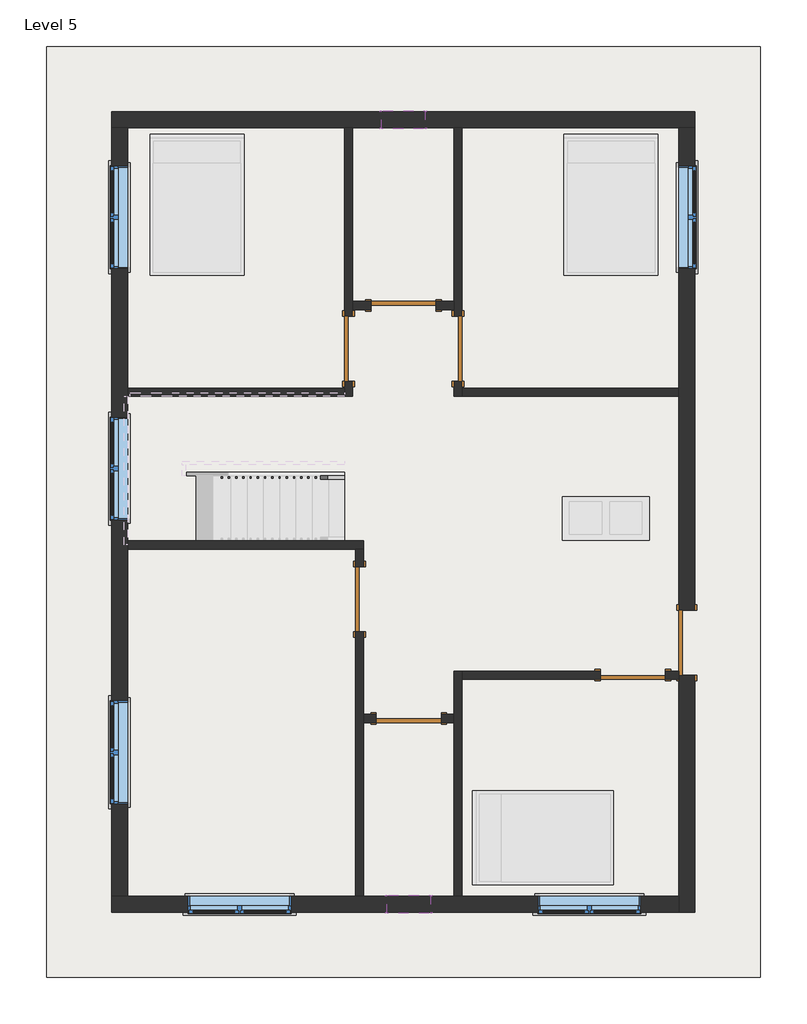
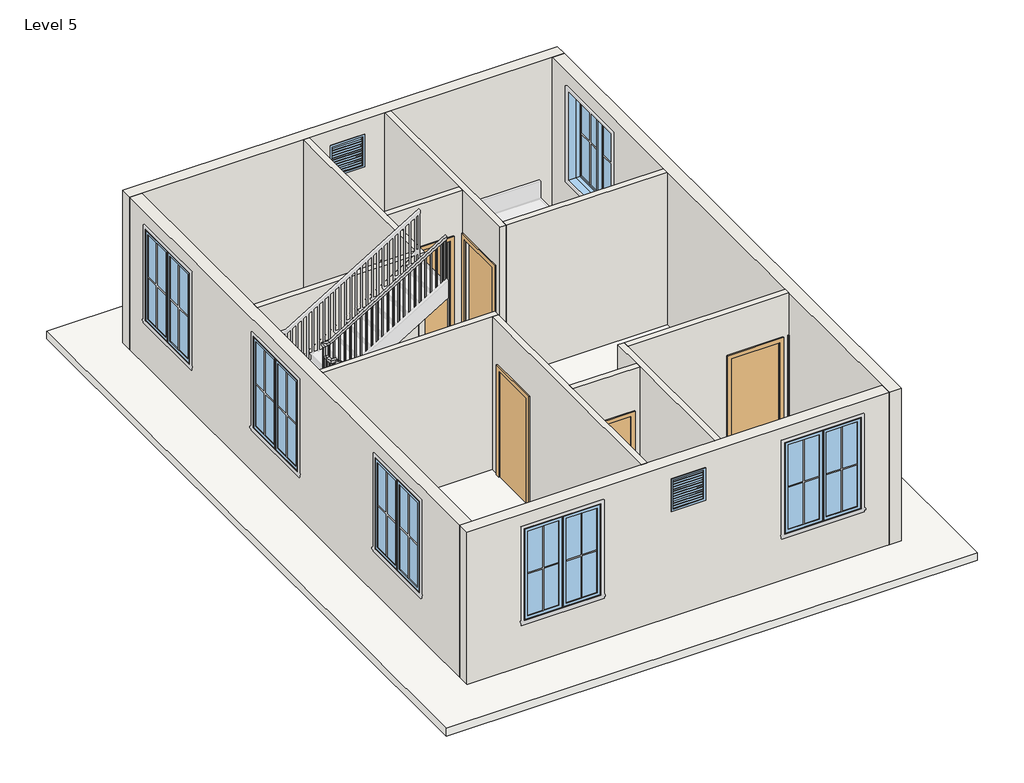
# One storey, part 1 of 2: 14 walls, 8 windows, 7 doors, 1 railing, 1 roof, 1 slab.
"""IFC4 building model written with IfcOpenShell, lengths in millimetres."""

from ifc_helpers import new_model, si_unit, frame, origin, place, context, project, spatial, polyline, outline, extrude, faceted_brep, transform, mapped, element, save
from components import door_305aa2a5, door_e5f9f3c4, door_0ca8825f, window_9ac97e1a, window_f2d8fef0

model = new_model("IFC4")

# Units and contexts
model_context = context("Model", 3, world=origin())
ifc_project = project(units=[si_unit("LENGTHUNIT", "METRE", prefix="MILLI")], contexts=[model_context])

# Site, building, storey
site = spatial("IfcSite", under=ifc_project)
building = spatial("IfcBuilding", under=site)
storey = spatial("IfcBuildingStorey", under=building, Name="Level 5", Elevation=9601.2)

# Doors
placement = place(None, origin())
door_shape = door_305aa2a5(model_context)
element("IfcDoor", 1, ObjectType="Single-Flush : 36\" x 84\"", at=placement, inside=storey, context=model_context, shape_type="MappedRepresentation", body=[
    mapped(door_shape, transform((-2023.6910855, 2116.5303617, 9601.2), x_axis=(0.0, -1.0, 0.0), y_axis=(1.0, 0.0, 0.0), z_axis=(0.0, 0.0, 1.0))),
])
element("IfcDoor", 2, ObjectType="Single-Flush : 36\" x 84\"", at=placement, inside=storey, context=model_context, shape_type="MappedRepresentation", body=[
    mapped(door_shape, transform((-1179.1410855, -3078.1725945, 9601.2), x_axis=(1.0, 0.0, 0.0), y_axis=(0.0, 1.0, 0.0), z_axis=(0.0, 0.0, 1.0))),
])
element("IfcDoor", 3, ObjectType="Single-Flush : 36\" x 84\"", at=placement, inside=storey, context=model_context, shape_type="MappedRepresentation", body=[
    mapped(door_shape, transform((1970.4589145, -2468.1696383, 9601.2), x_axis=(1.0, 0.0, 0.0), y_axis=(0.0, 1.0, 0.0), z_axis=(0.0, 0.0, 1.0))),
])
door_2_shape = door_e5f9f3c4(model_context)
element("IfcDoor", 4, ObjectType="Single-Flush : 36\" x 84\"", at=placement, inside=storey, context=model_context, shape_type="MappedRepresentation", body=[
    mapped(door_2_shape, transform((-486.9910855, 2116.5303617, 9601.2), x_axis=(0.0, -1.0, 0.0), y_axis=(1.0, 0.0, 0.0), z_axis=(0.0, 0.0, 1.0))),
])
element("IfcDoor", 5, ObjectType="Single-Flush : 36\" x 84\"", at=placement, inside=storey, context=model_context, shape_type="MappedRepresentation", body=[
    mapped(door_2_shape, transform((-1871.2910855, -1401.3696383, 9601.2), x_axis=(0.0, 1.0, 0.0), y_axis=(-1.0, 0.0, 0.0), z_axis=(0.0, 0.0, 1.0))),
])
element("IfcDoor", 6, ObjectType="Single-Flush : 36\" x 84\"", at=placement, inside=storey, context=model_context, shape_type="MappedRepresentation", body=[
    mapped(door_2_shape, transform((-1255.3410855, 2726.1303617, 9601.2), x_axis=(1.0, 0.0, 0.0), y_axis=(0.0, 1.0, 0.0), z_axis=(0.0, 0.0, 1.0))),
])
door_3_shape = door_0ca8825f(model_context)
element("IfcDoor", 7, ObjectType="Single-Flush : 36\" x 84\"", at=placement, inside=storey, context=model_context, shape_type="MappedRepresentation", body=[
    mapped(door_3_shape, transform((2732.4589145, -2010.9696383, 9601.2), x_axis=(0.0, 1.0, 0.0), y_axis=(-1.0, 0.0, 0.0), z_axis=(0.0, 0.0, 1.0))),
])

# Railing
element("IfcRailing", 8, ObjectType="Handrail - Rectangular", at=placement, inside=storey, context=model_context, shape_type="SolidModel", body=[
    faceted_brep([(-2080.8410855, 281.3803617, 10654.1454545), (-2080.8410855, 281.3803617, 10594.7439943), (-2080.8410855, 332.1803617, 10594.7439943), (-2080.8410855, 332.1803617, 10654.1454545), (-4290.6410855, 281.3803617, 11993.4181818), (-4341.4410855, 281.3803617, 11964.8046004), (-4341.4410855, 332.1803617, 11964.8046004), (-4290.6410855, 332.1803617, 11993.4181818), (-4290.6410855, 281.3803617, 12039.6), (-4341.4410855, 281.3803617, 11988.8), (-4341.4410855, 332.1803617, 11988.8), (-4290.6410855, 332.1803617, 12039.6), (-4417.6410855, 281.3803617, 12039.6), (-4417.6410855, 281.3803617, 11988.8), (-4366.8410855, 332.1803617, 11988.8), (-4366.8410855, 332.1803617, 12039.6), (-4417.6410855, 408.3803617, 12039.6), (-4417.6410855, 408.3803617, 11988.8), (-4366.8410855, 408.3803617, 11988.8), (-4366.8410855, 408.3803617, 12039.6), (-4417.6410855, 459.1803617, 12039.6), (-4417.6410855, 509.9803617, 11988.8), (-4366.8410855, 509.9803617, 11988.8), (-4366.8410855, 459.1803617, 12039.6), (-4417.6410855, 459.1803617, 12224.3272727), (-4417.6410855, 509.9803617, 12173.5272727), (-4366.8410855, 509.9803617, 12173.5272727), (-4366.8410855, 459.1803617, 12224.3272727), (-4417.6410855, 586.1803617, 12224.3272727), (-4417.6410855, 586.1803617, 12173.5272727), (-4366.8410855, 535.3803617, 12173.5272727), (-4366.8410855, 535.3803617, 12224.3272727), (-4290.6410855, 586.1803617, 12224.3272727), (-4276.4486761, 586.1803617, 12173.5272727), (-4276.4486761, 535.3803617, 12173.5272727), (-4290.6410855, 535.3803617, 12224.3272727), (-2080.8410855, 586.1803617, 13563.6), (-2080.8410855, 535.3803617, 13563.6), (-2080.8410855, 535.3803617, 13504.1985397), (-2080.8410855, 586.1803617, 13504.1985397)], [[[0, 1, 2, 3]], [[1, 0, 4, 5]], [[2, 1, 5, 6]], [[3, 2, 6, 7]], [[0, 3, 7, 4]], [[5, 4, 8, 9]], [[6, 5, 9, 10]], [[7, 6, 10, 11]], [[4, 7, 11, 8]], [[9, 8, 12, 13]], [[10, 9, 13, 14]], [[11, 10, 14, 15]], [[8, 11, 15, 12]], [[13, 12, 16, 17]], [[14, 13, 17, 18]], [[15, 14, 18, 19]], [[12, 15, 19, 16]], [[17, 16, 20, 21]], [[18, 17, 21, 22]], [[19, 18, 22, 23]], [[16, 19, 23, 20]], [[21, 20, 24, 25]], [[22, 21, 25, 26]], [[23, 22, 26, 27]], [[20, 23, 27, 24]], [[25, 24, 28, 29]], [[26, 25, 29, 30]], [[27, 26, 30, 31]], [[24, 27, 31, 28]], [[29, 28, 32, 33]], [[30, 29, 33, 34]], [[31, 30, 34, 35]], [[28, 31, 35, 32]], [[36, 37, 38, 39]], [[33, 32, 36, 39]], [[34, 33, 39, 38]], [[35, 34, 38, 37]], [[32, 35, 37, 36]]]),
    extrude(outline(polyline([(13463.7894488, -2147.5160855), (13452.2439943, -2166.5660855), (12510.6545455, -2166.5660855), (12510.6545455, -2147.5160855), (13463.7894488, -2147.5160855)])), frame((0.0, 551.2553617, 0.0), z_axis=(0.0, 1.0, 0.0), x_axis=(0.0, 0.0, 1.0)), (0.0, 0.0, 1.0), 19.05),
    extrude(outline(polyline([(13402.2136913, -2249.1160855), (13390.6682367, -2268.1660855), (12510.6545455, -2268.1660855), (12510.6545455, -2249.1160855), (13402.2136913, -2249.1160855)])), frame((0.0, 551.2553617, 0.0), z_axis=(0.0, 1.0, 0.0), x_axis=(0.0, 0.0, 1.0)), (0.0, 0.0, 1.0), 19.05),
    extrude(outline(polyline([(13340.6379337, -2350.7160855), (13329.0924791, -2369.7660855), (12372.1090909, -2369.7660855), (12372.1090909, -2350.7160855), (13340.6379337, -2350.7160855)])), frame((0.0, 551.2553617, 0.0), z_axis=(0.0, 1.0, 0.0), x_axis=(0.0, 0.0, 1.0)), (0.0, 0.0, 1.0), 19.05),
    extrude(outline(polyline([(13279.0621761, -2452.3160855), (13267.5167216, -2471.3660855), (12372.1090909, -2471.3660855), (12372.1090909, -2452.3160855), (13279.0621761, -2452.3160855)])), frame((0.0, 551.2553617, 0.0), z_axis=(0.0, 1.0, 0.0), x_axis=(0.0, 0.0, 1.0)), (0.0, 0.0, 1.0), 19.05),
    extrude(outline(polyline([(13217.4864185, -2553.9160855), (13205.940964, -2572.9660855), (12233.5636364, -2572.9660855), (12233.5636364, -2553.9160855), (13217.4864185, -2553.9160855)])), frame((0.0, 551.2553617, 0.0), z_axis=(0.0, 1.0, 0.0), x_axis=(0.0, 0.0, 1.0)), (0.0, 0.0, 1.0), 19.05),
    extrude(outline(polyline([(13155.910661, -2655.5160855), (13144.3652064, -2674.5660855), (12233.5636364, -2674.5660855), (12233.5636364, -2655.5160855), (13155.910661, -2655.5160855)])), frame((0.0, 551.2553617, 0.0), z_axis=(0.0, 1.0, 0.0), x_axis=(0.0, 0.0, 1.0)), (0.0, 0.0, 1.0), 19.05),
    extrude(outline(polyline([(13094.3349034, -2757.1160855), (13082.7894488, -2776.1660855), (12233.5636364, -2776.1660855), (12233.5636364, -2757.1160855), (13094.3349034, -2757.1160855)])), frame((0.0, 551.2553617, 0.0), z_axis=(0.0, 1.0, 0.0), x_axis=(0.0, 0.0, 1.0)), (0.0, 0.0, 1.0), 19.05),
    extrude(outline(polyline([(13032.7591458, -2858.7160855), (13021.2136913, -2877.7660855), (12095.0181818, -2877.7660855), (12095.0181818, -2858.7160855), (13032.7591458, -2858.7160855)])), frame((0.0, 551.2553617, 0.0), z_axis=(0.0, 1.0, 0.0), x_axis=(0.0, 0.0, 1.0)), (0.0, 0.0, 1.0), 19.05),
    extrude(outline(polyline([(12971.1833882, -2960.3160855), (12959.6379337, -2979.3660855), (12095.0181818, -2979.3660855), (12095.0181818, -2960.3160855), (12971.1833882, -2960.3160855)])), frame((0.0, 551.2553617, 0.0), z_axis=(0.0, 1.0, 0.0), x_axis=(0.0, 0.0, 1.0)), (0.0, 0.0, 1.0), 19.05),
    extrude(outline(polyline([(12909.6076307, -3061.9160855), (12898.0621761, -3080.9660855), (11956.4727273, -3080.9660855), (11956.4727273, -3061.9160855), (12909.6076307, -3061.9160855)])), frame((0.0, 551.2553617, 0.0), z_axis=(0.0, 1.0, 0.0), x_axis=(0.0, 0.0, 1.0)), (0.0, 0.0, 1.0), 19.05),
    extrude(outline(polyline([(12848.0318731, -3163.5160855), (12836.4864185, -3182.5660855), (11956.4727273, -3182.5660855), (11956.4727273, -3163.5160855), (12848.0318731, -3163.5160855)])), frame((0.0, 551.2553617, 0.0), z_axis=(0.0, 1.0, 0.0), x_axis=(0.0, 0.0, 1.0)), (0.0, 0.0, 1.0), 19.05),
    extrude(outline(polyline([(12786.4561155, -3265.1160855), (12774.910661, -3284.1660855), (11817.9272727, -3284.1660855), (11817.9272727, -3265.1160855), (12786.4561155, -3265.1160855)])), frame((0.0, 551.2553617, 0.0), z_axis=(0.0, 1.0, 0.0), x_axis=(0.0, 0.0, 1.0)), (0.0, 0.0, 1.0), 19.05),
    extrude(outline(polyline([(12724.8803579, -3366.7160855), (12713.3349034, -3385.7660855), (11817.9272727, -3385.7660855), (11817.9272727, -3366.7160855), (12724.8803579, -3366.7160855)])), frame((0.0, 551.2553617, 0.0), z_axis=(0.0, 1.0, 0.0), x_axis=(0.0, 0.0, 1.0)), (0.0, 0.0, 1.0), 19.05),
    extrude(outline(polyline([(12663.3046004, -3468.3160855), (12651.7591458, -3487.3660855), (11679.3818182, -3487.3660855), (11679.3818182, -3468.3160855), (12663.3046004, -3468.3160855)])), frame((0.0, 551.2553617, 0.0), z_axis=(0.0, 1.0, 0.0), x_axis=(0.0, 0.0, 1.0)), (0.0, 0.0, 1.0), 19.05),
    extrude(outline(polyline([(12601.7288428, -3569.9160855), (12590.1833882, -3588.9660855), (11679.3818182, -3588.9660855), (11679.3818182, -3569.9160855), (12601.7288428, -3569.9160855)])), frame((0.0, 551.2553617, 0.0), z_axis=(0.0, 1.0, 0.0), x_axis=(0.0, 0.0, 1.0)), (0.0, 0.0, 1.0), 19.05),
    extrude(outline(polyline([(12540.1530852, -3671.5160855), (12528.6076307, -3690.5660855), (11679.3818182, -3690.5660855), (11679.3818182, -3671.5160855), (12540.1530852, -3671.5160855)])), frame((0.0, 551.2553617, 0.0), z_axis=(0.0, 1.0, 0.0), x_axis=(0.0, 0.0, 1.0)), (0.0, 0.0, 1.0), 19.05),
    extrude(outline(polyline([(12478.5773276, -3773.1160855), (12467.0318731, -3792.1660855), (11540.8363636, -3792.1660855), (11540.8363636, -3773.1160855), (12478.5773276, -3773.1160855)])), frame((0.0, 551.2553617, 0.0), z_axis=(0.0, 1.0, 0.0), x_axis=(0.0, 0.0, 1.0)), (0.0, 0.0, 1.0), 19.05),
    extrude(outline(polyline([(12417.00157, -3874.7160855), (12405.4561155, -3893.7660855), (11540.8363636, -3893.7660855), (11540.8363636, -3874.7160855), (12417.00157, -3874.7160855)])), frame((0.0, 551.2553617, 0.0), z_axis=(0.0, 1.0, 0.0), x_axis=(0.0, 0.0, 1.0)), (0.0, 0.0, 1.0), 19.05),
    extrude(outline(polyline([(12355.4258125, -3976.3160855), (12343.8803579, -3995.3660855), (11402.2909091, -3995.3660855), (11402.2909091, -3976.3160855), (12355.4258125, -3976.3160855)])), frame((0.0, 551.2553617, 0.0), z_axis=(0.0, 1.0, 0.0), x_axis=(0.0, 0.0, 1.0)), (0.0, 0.0, 1.0), 19.05),
    extrude(outline(polyline([(12293.8500549, -4077.9160855), (12282.3046004, -4096.9660855), (11402.2909091, -4096.9660855), (11402.2909091, -4077.9160855), (12293.8500549, -4077.9160855)])), frame((0.0, 551.2553617, 0.0), z_axis=(0.0, 1.0, 0.0), x_axis=(0.0, 0.0, 1.0)), (0.0, 0.0, 1.0), 19.05),
    extrude(outline(polyline([(12232.2742973, -4179.5160855), (12220.7288428, -4198.5660855), (11263.7454545, -4198.5660855), (11263.7454545, -4179.5160855), (12232.2742973, -4179.5160855)])), frame((0.0, 551.2553617, 0.0), z_axis=(0.0, 1.0, 0.0), x_axis=(0.0, 0.0, 1.0)), (0.0, 0.0, 1.0), 19.05),
    extrude(outline(polyline([(12170.6985397, -4281.1160855), (12159.1530852, -4300.1660855), (11263.7454545, -4300.1660855), (11263.7454545, -4281.1160855), (12170.6985397, -4281.1160855)])), frame((0.0, 551.2553617, 0.0), z_axis=(0.0, 1.0, 0.0), x_axis=(0.0, 0.0, 1.0)), (0.0, 0.0, 1.0), 19.05),
    extrude(outline(polyline([(-4382.7160855, 500.4553617), (-4401.7660855, 500.4553617), (-4401.7660855, 519.5053617), (-4382.7160855, 519.5053617), (-4382.7160855, 500.4553617)])), frame((0.0, 0.0, 11125.2), z_axis=(0.0, 0.0, 1.0), x_axis=(1.0, 0.0, 0.0)), (0.0, 0.0, 1.0), 1048.3272727),
    extrude(outline(polyline([(-4382.7160855, 398.8553617), (-4401.7660855, 398.8553617), (-4401.7660855, 417.9053617), (-4382.7160855, 417.9053617), (-4382.7160855, 398.8553617)])), frame((0.0, 0.0, 11125.2), z_axis=(0.0, 0.0, 1.0), x_axis=(1.0, 0.0, 0.0)), (0.0, 0.0, 1.0), 863.6),
    extrude(outline(polyline([(-4306.5160855, 316.3053617), (-4306.5160855, 297.2553617), (-4325.5660855, 297.2553617), (-4325.5660855, 316.3053617), (-4306.5160855, 316.3053617)])), frame((0.0, 0.0, 10986.6545455), z_axis=(0.0, 0.0, 1.0), x_axis=(1.0, 0.0, 0.0)), (0.0, 0.0, 1.0), 1002.1454545),
    extrude(outline(polyline([(11882.0621761, -4204.9160855), (11893.6076307, -4223.9660855), (10986.6545455, -4223.9660855), (10986.6545455, -4204.9160855), (11882.0621761, -4204.9160855)])), frame((0.0, 297.2553617, 0.0), z_axis=(0.0, 1.0, 0.0), x_axis=(0.0, 0.0, 1.0)), (0.0, 0.0, 1.0), 19.05),
    extrude(outline(polyline([(11820.4864185, -4103.3160855), (11832.0318731, -4122.3660855), (10848.1090909, -4122.3660855), (10848.1090909, -4103.3160855), (11820.4864185, -4103.3160855)])), frame((0.0, 297.2553617, 0.0), z_axis=(0.0, 1.0, 0.0), x_axis=(0.0, 0.0, 1.0)), (0.0, 0.0, 1.0), 19.05),
    extrude(outline(polyline([(11758.910661, -4001.7160855), (11770.4561155, -4020.7660855), (10848.1090909, -4020.7660855), (10848.1090909, -4001.7160855), (11758.910661, -4001.7160855)])), frame((0.0, 297.2553617, 0.0), z_axis=(0.0, 1.0, 0.0), x_axis=(0.0, 0.0, 1.0)), (0.0, 0.0, 1.0), 19.05),
    extrude(outline(polyline([(11697.3349034, -3900.1160855), (11708.8803579, -3919.1660855), (10848.1090909, -3919.1660855), (10848.1090909, -3900.1160855), (11697.3349034, -3900.1160855)])), frame((0.0, 297.2553617, 0.0), z_axis=(0.0, 1.0, 0.0), x_axis=(0.0, 0.0, 1.0)), (0.0, 0.0, 1.0), 19.05),
    extrude(outline(polyline([(11635.7591458, -3798.5160855), (11647.3046004, -3817.5660855), (10709.5636364, -3817.5660855), (10709.5636364, -3798.5160855), (11635.7591458, -3798.5160855)])), frame((0.0, 297.2553617, 0.0), z_axis=(0.0, 1.0, 0.0), x_axis=(0.0, 0.0, 1.0)), (0.0, 0.0, 1.0), 19.05),
    extrude(outline(polyline([(11574.1833882, -3696.9160855), (11585.7288428, -3715.9660855), (10709.5636364, -3715.9660855), (10709.5636364, -3696.9160855), (11574.1833882, -3696.9160855)])), frame((0.0, 297.2553617, 0.0), z_axis=(0.0, 1.0, 0.0), x_axis=(0.0, 0.0, 1.0)), (0.0, 0.0, 1.0), 19.05),
    extrude(outline(polyline([(11512.6076307, -3595.3160855), (11524.1530852, -3614.3660855), (10571.0181818, -3614.3660855), (10571.0181818, -3595.3160855), (11512.6076307, -3595.3160855)])), frame((0.0, 297.2553617, 0.0), z_axis=(0.0, 1.0, 0.0), x_axis=(0.0, 0.0, 1.0)), (0.0, 0.0, 1.0), 19.05),
    extrude(outline(polyline([(11451.0318731, -3493.7160855), (11462.5773276, -3512.7660855), (10571.0181818, -3512.7660855), (10571.0181818, -3493.7160855), (11451.0318731, -3493.7160855)])), frame((0.0, 297.2553617, 0.0), z_axis=(0.0, 1.0, 0.0), x_axis=(0.0, 0.0, 1.0)), (0.0, 0.0, 1.0), 19.05),
    extrude(outline(polyline([(11389.4561155, -3392.1160855), (11401.00157, -3411.1660855), (10432.4727273, -3411.1660855), (10432.4727273, -3392.1160855), (11389.4561155, -3392.1160855)])), frame((0.0, 297.2553617, 0.0), z_axis=(0.0, 1.0, 0.0), x_axis=(0.0, 0.0, 1.0)), (0.0, 0.0, 1.0), 19.05),
    extrude(outline(polyline([(11327.8803579, -3290.5160855), (11339.4258125, -3309.5660855), (10432.4727273, -3309.5660855), (10432.4727273, -3290.5160855), (11327.8803579, -3290.5160855)])), frame((0.0, 297.2553617, 0.0), z_axis=(0.0, 1.0, 0.0), x_axis=(0.0, 0.0, 1.0)), (0.0, 0.0, 1.0), 19.05),
    extrude(outline(polyline([(11266.3046004, -3188.9160855), (11277.8500549, -3207.9660855), (10293.9272727, -3207.9660855), (10293.9272727, -3188.9160855), (11266.3046004, -3188.9160855)])), frame((0.0, 297.2553617, 0.0), z_axis=(0.0, 1.0, 0.0), x_axis=(0.0, 0.0, 1.0)), (0.0, 0.0, 1.0), 19.05),
    extrude(outline(polyline([(11204.7288428, -3087.3160855), (11216.2742973, -3106.3660855), (10293.9272727, -3106.3660855), (10293.9272727, -3087.3160855), (11204.7288428, -3087.3160855)])), frame((0.0, 297.2553617, 0.0), z_axis=(0.0, 1.0, 0.0), x_axis=(0.0, 0.0, 1.0)), (0.0, 0.0, 1.0), 19.05),
    extrude(outline(polyline([(11143.1530852, -2985.7160855), (11154.6985397, -3004.7660855), (10293.9272727, -3004.7660855), (10293.9272727, -2985.7160855), (11143.1530852, -2985.7160855)])), frame((0.0, 297.2553617, 0.0), z_axis=(0.0, 1.0, 0.0), x_axis=(0.0, 0.0, 1.0)), (0.0, 0.0, 1.0), 19.05),
    extrude(outline(polyline([(11081.5773276, -2884.1160855), (11093.1227822, -2903.1660855), (10155.3818182, -2903.1660855), (10155.3818182, -2884.1160855), (11081.5773276, -2884.1160855)])), frame((0.0, 297.2553617, 0.0), z_axis=(0.0, 1.0, 0.0), x_axis=(0.0, 0.0, 1.0)), (0.0, 0.0, 1.0), 19.05),
    extrude(outline(polyline([(11020.00157, -2782.5160855), (11031.5470246, -2801.5660855), (10155.3818182, -2801.5660855), (10155.3818182, -2782.5160855), (11020.00157, -2782.5160855)])), frame((0.0, 297.2553617, 0.0), z_axis=(0.0, 1.0, 0.0), x_axis=(0.0, 0.0, 1.0)), (0.0, 0.0, 1.0), 19.05),
    extrude(outline(polyline([(10958.4258125, -2680.9160855), (10969.971267, -2699.9660855), (10016.8363636, -2699.9660855), (10016.8363636, -2680.9160855), (10958.4258125, -2680.9160855)])), frame((0.0, 297.2553617, 0.0), z_axis=(0.0, 1.0, 0.0), x_axis=(0.0, 0.0, 1.0)), (0.0, 0.0, 1.0), 19.05),
    extrude(outline(polyline([(10896.8500549, -2579.3160855), (10908.3955094, -2598.3660855), (10016.8363636, -2598.3660855), (10016.8363636, -2579.3160855), (10896.8500549, -2579.3160855)])), frame((0.0, 297.2553617, 0.0), z_axis=(0.0, 1.0, 0.0), x_axis=(0.0, 0.0, 1.0)), (0.0, 0.0, 1.0), 19.05),
    extrude(outline(polyline([(10835.2742973, -2477.7160855), (10846.8197519, -2496.7660855), (9878.2909091, -2496.7660855), (9878.2909091, -2477.7160855), (10835.2742973, -2477.7160855)])), frame((0.0, 297.2553617, 0.0), z_axis=(0.0, 1.0, 0.0), x_axis=(0.0, 0.0, 1.0)), (0.0, 0.0, 1.0), 19.05),
    extrude(outline(polyline([(10773.6985397, -2376.1160855), (10785.2439943, -2395.1660855), (9878.2909091, -2395.1660855), (9878.2909091, -2376.1160855), (10773.6985397, -2376.1160855)])), frame((0.0, 297.2553617, 0.0), z_axis=(0.0, 1.0, 0.0), x_axis=(0.0, 0.0, 1.0)), (0.0, 0.0, 1.0), 19.05),
    extrude(outline(polyline([(10712.1227822, -2274.5160855), (10723.6682367, -2293.5660855), (9739.7454545, -2293.5660855), (9739.7454545, -2274.5160855), (10712.1227822, -2274.5160855)])), frame((0.0, 297.2553617, 0.0), z_axis=(0.0, 1.0, 0.0), x_axis=(0.0, 0.0, 1.0)), (0.0, 0.0, 1.0), 19.05),
    extrude(outline(polyline([(10650.5470246, -2172.9160855), (10662.0924791, -2191.9660855), (9739.7454545, -2191.9660855), (9739.7454545, -2172.9160855), (10650.5470246, -2172.9160855)])), frame((0.0, 297.2553617, 0.0), z_axis=(0.0, 1.0, 0.0), x_axis=(0.0, 0.0, 1.0)), (0.0, 0.0, 1.0), 19.05),
    extrude(outline(polyline([(-4382.7160855, 551.2553617), (-4401.7660855, 551.2553617), (-4401.7660855, 570.3053617), (-4382.7160855, 570.3053617), (-4382.7160855, 551.2553617)])), frame((0.0, 0.0, 11125.2), z_axis=(0.0, 0.0, 1.0), x_axis=(1.0, 0.0, 0.0)), (0.0, 0.0, 1.0), 1048.3272727),
    extrude(outline(polyline([(-4382.7160855, 316.3053617), (-4382.7160855, 297.2553617), (-4401.7660855, 297.2553617), (-4401.7660855, 316.3053617), (-4382.7160855, 316.3053617)])), frame((0.0, 0.0, 11125.2), z_axis=(0.0, 0.0, 1.0), x_axis=(1.0, 0.0, 0.0)), (0.0, 0.0, 1.0), 863.6),
    extrude(outline(polyline([(13504.1985397, -2080.8410855), (13492.6530852, -2099.8910855), (12510.6545455, -2099.8910855), (12510.6545455, -2080.8410855), (13504.1985397, -2080.8410855)])), frame((0.0, 551.2553617, 0.0), z_axis=(0.0, 1.0, 0.0), x_axis=(0.0, 0.0, 1.0)), (0.0, 0.0, 1.0), 19.05),
    extrude(outline(polyline([(10594.7439943, -2080.8410855), (10606.2894488, -2099.8910855), (9739.7454545, -2099.8910855), (9739.7454545, -2080.8410855), (10594.7439943, -2080.8410855)])), frame((0.0, 297.2553617, 0.0), z_axis=(0.0, 1.0, 0.0), x_axis=(0.0, 0.0, 1.0)), (0.0, 0.0, 1.0), 19.05),
])

# Roof
element("IfcRoof", 9, ObjectType="ROOF 6\"", at=placement, inside=storey, context=model_context, shape_type="SweptSolid", body=[
    extrude(outline(polyline([(-6271.8410855, 6364.6803617), (3761.1589145, 6364.6803617), (3761.1589145, -6716.3196383), (-6271.8410855, -6716.3196383), (-6271.8410855, 6364.6803617)])), frame((0.0, 0.0, 9448.8), z_axis=(0.0, 0.0, 1.0), x_axis=(1.0, 0.0, 0.0)), (0.0, 0.0, 1.0), 152.4),
])

# Slab
element("IfcSlab", 10, ObjectType="FLOOR 6\"", at=placement, inside=storey, context=model_context, shape_type="SweptSolid", body=[
    extrude(outline(polyline([(2846.7589145, 5450.2803617), (2846.7589145, -5801.9196383), (-5357.4410855, -5801.9196383), (-5357.4410855, 5450.2803617), (2846.7589145, 5450.2803617)])), frame((0.0, 0.0, 9448.8), z_axis=(0.0, 0.0, 1.0), x_axis=(1.0, 0.0, 0.0)), (0.0, 0.0, 1.0), 152.4),
])

# Walls
element("IfcWall", 11, ObjectType="WALL 4.5\"", at=placement, inside=storey, context=model_context, shape_type="Brep", body=[
    faceted_brep([(-2080.8410855, 1659.3303617, 11734.8), (-2080.8410855, 1659.3303617, 9601.2), (-2080.8410855, 1564.0803617, 9601.2), (-2080.8410855, 1449.7803617, 9601.2), (-2080.8410855, 1449.7803617, 12649.2), (-2080.8410855, 1564.0803617, 12649.2), (-2080.8410855, 5221.6803617, 12649.2), (-2080.8410855, 5221.6803617, 9601.2), (-2080.8410855, 2573.7303617, 9601.2), (-2080.8410855, 2573.7303617, 11734.8), (-1966.5410855, 1449.7803617, 9601.2), (-1966.5410855, 1659.3303617, 9601.2), (-1966.5410855, 1659.3303617, 11734.8), (-1966.5410855, 2573.7303617, 11734.8), (-1966.5410855, 2573.7303617, 9601.2), (-1966.5410855, 2668.9803617, 9601.2), (-1966.5410855, 2783.2803617, 9601.2), (-1966.5410855, 5221.6803617, 9601.2), (-1966.5410855, 5221.6803617, 12649.2), (-1966.5410855, 2783.2803617, 12649.2), (-1966.5410855, 2668.9803617, 12649.2), (-1966.5410855, 1449.7803617, 12649.2)], [[[0, 1, 2, 3, 4, 5, 6, 7, 8, 9]], [[10, 11, 12, 13, 14, 15, 16, 17, 18, 19, 20, 21]], [[8, 7, 17, 16, 15, 14]], [[3, 2, 1, 11, 10]], [[7, 6, 18, 17]], [[4, 3, 10, 21]], [[12, 11, 1, 0]], [[13, 12, 0, 9]], [[14, 13, 9, 8]], [[6, 5, 4, 21, 20, 19, 18]]]),
])
element("IfcWall", 12, ObjectType="WALL 4.5\"", at=placement, inside=storey, context=model_context, shape_type="SweptSolid", body=[
    extrude(outline(polyline([(-5128.8410855, 1564.0803617), (-2080.8410855, 1564.0803617), (-2080.8410855, 1449.7803617), (-5128.8410855, 1449.7803617), (-5128.8410855, 1564.0803617)])), frame((0.0, 0.0, 9601.2), z_axis=(0.0, 0.0, 1.0), x_axis=(1.0, 0.0, 0.0)), (0.0, 0.0, 1.0), 3048.0),
])
element("IfcWall", 13, ObjectType="WALL 4.5\"", at=placement, inside=storey, context=model_context, shape_type="Brep", body=[
    faceted_brep([(-544.1410855, 1659.3303617, 11734.8), (-544.1410855, 1659.3303617, 9601.2), (-544.1410855, 1449.7803617, 9601.2), (-544.1410855, 1449.7803617, 12649.2), (-544.1410855, 2668.9803617, 12649.2), (-544.1410855, 2783.2803617, 12649.2), (-544.1410855, 5221.6803617, 12649.2), (-544.1410855, 5221.6803617, 9601.2), (-544.1410855, 2783.2803617, 9601.2), (-544.1410855, 2668.9803617, 9601.2), (-544.1410855, 2573.7303617, 9601.2), (-544.1410855, 2573.7303617, 11734.8), (-429.8410855, 1449.7803617, 9601.2), (-429.8410855, 1564.0803617, 9601.2), (-429.8410855, 1659.3303617, 9601.2), (-429.8410855, 1659.3303617, 11734.8), (-429.8410855, 2573.7303617, 11734.8), (-429.8410855, 2573.7303617, 9601.2), (-429.8410855, 5221.6803617, 9601.2), (-429.8410855, 5221.6803617, 12649.2), (-429.8410855, 1564.0803617, 12649.2), (-429.8410855, 1449.7803617, 12649.2)], [[[0, 1, 2, 3, 4, 5, 6, 7, 8, 9, 10, 11]], [[12, 13, 14, 15, 16, 17, 18, 19, 20, 21]], [[2, 1, 14, 13, 12]], [[10, 9, 8, 7, 18, 17]], [[7, 6, 19, 18]], [[3, 2, 12, 21]], [[15, 14, 1, 0]], [[16, 15, 0, 11]], [[17, 16, 11, 10]], [[6, 5, 4, 3, 21, 20, 19]]]),
])
element("IfcWall", 14, ObjectType="WALL 4.5\"", at=placement, inside=storey, context=model_context, shape_type="SweptSolid", body=[
    extrude(outline(polyline([(2618.1589145, 1449.7803617), (-429.8410855, 1449.7803617), (-429.8410855, 1564.0803617), (2618.1589145, 1564.0803617), (2618.1589145, 1449.7803617)])), frame((0.0, 0.0, 9601.2), z_axis=(0.0, 0.0, 1.0), x_axis=(1.0, 0.0, 0.0)), (0.0, 0.0, 1.0), 3048.0),
])
element("IfcWall", 15, ObjectType="WALL 4.5\"", at=placement, inside=storey, context=model_context, shape_type="Brep", body=[
    faceted_brep([(-5128.8410855, -696.5196383, 9601.2), (-1928.4410855, -696.5196383, 9601.2), (-1814.1410855, -696.5196383, 9601.2), (-1814.1410855, -696.5196383, 12649.2), (-1928.4410855, -696.5196383, 12649.2), (-5128.8410855, -696.5196383, 12649.2), (-5128.8410855, -582.2196383, 9601.2), (-5128.8410855, -582.2196383, 12649.2), (-1814.1410855, -582.2196383, 12649.2), (-1814.1410855, -582.2196383, 9601.2)], [[[0, 1, 2, 3, 4, 5]], [[6, 7, 8, 9]], [[2, 1, 0, 6, 9]], [[0, 5, 7, 6]], [[3, 2, 9, 8]], [[5, 4, 3, 8, 7]]]),
])
element("IfcWall", 16, ObjectType="WALL 4.5\"", at=placement, inside=storey, context=model_context, shape_type="Brep", body=[
    faceted_brep([(-1814.1410855, -944.1696383, 11734.8), (-1814.1410855, -944.1696383, 9601.2), (-1814.1410855, -696.5196383, 9601.2), (-1814.1410855, -696.5196383, 12649.2), (-1814.1410855, -3021.0225945, 12649.2), (-1814.1410855, -3135.3225945, 12649.2), (-1814.1410855, -5573.3196383, 12649.2), (-1814.1410855, -5573.3196383, 9601.2), (-1814.1410855, -3135.3225945, 9601.2), (-1814.1410855, -3021.0225945, 9601.2), (-1814.1410855, -1858.5696383, 9601.2), (-1814.1410855, -1858.5696383, 11734.8), (-1928.4410855, -696.5196383, 9601.2), (-1928.4410855, -944.1696383, 9601.2), (-1928.4410855, -944.1696383, 11734.8), (-1928.4410855, -1858.5696383, 11734.8), (-1928.4410855, -1858.5696383, 9601.2), (-1928.4410855, -5573.3196383, 9601.2), (-1928.4410855, -5573.3196383, 12649.2), (-1928.4410855, -696.5196383, 12649.2)], [[[0, 1, 2, 3, 4, 5, 6, 7, 8, 9, 10, 11]], [[12, 13, 14, 15, 16, 17, 18, 19]], [[2, 1, 13, 12]], [[10, 9, 8, 7, 17, 16]], [[3, 2, 12, 19]], [[7, 6, 18, 17]], [[14, 13, 1, 0]], [[15, 14, 0, 11]], [[16, 15, 11, 10]], [[6, 5, 4, 3, 19, 18]]]),
])
element("IfcWall", 17, ObjectType="WALL 4.5\"", at=placement, inside=storey, context=model_context, shape_type="SweptSolid", body=[
    extrude(outline(polyline([(11734.8, -721.9410855), (9601.2, -721.9410855), (9601.2, -544.1410855), (12649.2, -544.1410855), (12649.2, -1814.1410855), (9601.2, -1814.1410855), (9601.2, -1636.3410855), (11734.8, -1636.3410855), (11734.8, -721.9410855)])), frame((0.0, -3135.3225945, 0.0), z_axis=(0.0, 1.0, 0.0), x_axis=(0.0, 0.0, 1.0)), (0.0, 0.0, 1.0), 114.3),
])
element("IfcWall", 18, ObjectType="WALL 4.5\"", at=placement, inside=storey, context=model_context, shape_type="Brep", body=[
    faceted_brep([(-544.1410855, -2411.0196383, 9601.2), (-544.1410855, -3021.0225945, 9601.2), (-544.1410855, -3135.3225945, 9601.2), (-544.1410855, -5573.3196383, 9601.2), (-544.1410855, -5573.3196383, 12649.2), (-544.1410855, -3135.3225945, 12649.2), (-544.1410855, -3021.0225945, 12649.2), (-544.1410855, -2411.0196383, 12649.2), (-429.8410855, -2411.0196383, 9601.2), (-429.8410855, -2411.0196383, 12649.2), (-429.8410855, -2525.3196383, 12649.2), (-429.8410855, -5573.3196383, 12649.2), (-429.8410855, -5573.3196383, 9601.2), (-429.8410855, -2525.3196383, 9601.2)], [[[0, 1, 2, 3, 4, 5, 6, 7]], [[8, 9, 10, 11, 12, 13]], [[3, 2, 1, 0, 8, 13, 12]], [[4, 3, 12, 11]], [[0, 7, 9, 8]], [[7, 6, 5, 4, 11, 10, 9]]]),
])
element("IfcWall", 19, ObjectType="WALL 4.5\"", at=placement, inside=storey, context=model_context, shape_type="Brep", body=[
    faceted_brep([(2427.6589145, -2525.3196383, 11734.8), (2427.6589145, -2525.3196383, 9601.2), (2618.1589145, -2525.3196383, 9601.2), (2618.1589145, -2525.3196383, 12649.2), (-429.8410855, -2525.3196383, 12649.2), (-429.8410855, -2525.3196383, 9601.2), (1513.2589145, -2525.3196383, 9601.2), (1513.2589145, -2525.3196383, 11734.8), (2618.1589145, -2411.0196383, 9601.2), (2427.6589145, -2411.0196383, 9601.2), (2427.6589145, -2411.0196383, 11734.8), (1513.2589145, -2411.0196383, 11734.8), (1513.2589145, -2411.0196383, 9601.2), (-429.8410855, -2411.0196383, 9601.2), (-429.8410855, -2411.0196383, 12649.2), (2618.1589145, -2411.0196383, 12649.2), (2618.1589145, -2468.1696383, 9601.2)], [[[0, 1, 2, 3, 4, 5, 6, 7]], [[8, 9, 10, 11, 12, 13, 14, 15]], [[6, 5, 13, 12]], [[2, 1, 9, 8, 16]], [[5, 4, 14, 13]], [[3, 2, 16, 8, 15]], [[10, 9, 1, 0]], [[11, 10, 0, 7]], [[12, 11, 7, 6]], [[4, 3, 15, 14]]]),
])
element("IfcWall", 20, ObjectType="WALL 4.5\"", at=placement, inside=storey, context=model_context, shape_type="SweptSolid", body=[
    extrude(outline(polyline([(11734.8, -798.1410855), (9601.2, -798.1410855), (9601.2, -544.1410855), (12649.2, -544.1410855), (12649.2, -1966.5410855), (9601.2, -1966.5410855), (9601.2, -1712.5410855), (11734.8, -1712.5410855), (11734.8, -798.1410855)])), frame((0.0, 2668.9803617, 0.0), z_axis=(0.0, 1.0, 0.0), x_axis=(0.0, 0.0, 1.0)), (0.0, 0.0, 1.0), 114.3),
])
element("IfcWall", 21, ObjectType="WALL 9\"", at=placement, inside=storey, context=model_context, shape_type="Brep", body=[
    faceted_brep([(-5357.4410855, 5221.6803617, 9601.2), (-5128.8410855, 5221.6803617, 9601.2), (-2080.8410855, 5221.6803617, 9601.2), (-1966.5410855, 5221.6803617, 9601.2), (-544.1410855, 5221.6803617, 9601.2), (-429.8410855, 5221.6803617, 9601.2), (2618.1589145, 5221.6803617, 9601.2), (2846.7589145, 5221.6803617, 9601.2), (2846.7589145, 5221.6803617, 12649.2), (2618.1589145, 5221.6803617, 12649.2), (-429.8410855, 5221.6803617, 12649.2), (-544.1410855, 5221.6803617, 12649.2), (-1966.5410855, 5221.6803617, 12649.2), (-2080.8410855, 5221.6803617, 12649.2), (-5128.8410855, 5221.6803617, 12649.2), (-5357.4410855, 5221.6803617, 12649.2), (-950.5410855, 5221.6803617, 12344.4), (-950.5410855, 5221.6803617, 11734.8), (-1560.1410855, 5221.6803617, 11734.8), (-1560.1410855, 5221.6803617, 12344.4), (-5357.4410855, 5450.2803617, 9601.2), (-5357.4410855, 5450.2803617, 12649.2), (2846.7589145, 5450.2803617, 12649.2), (2846.7589145, 5450.2803617, 9601.2), (-950.5410855, 5450.2803617, 12344.4), (-1560.1410855, 5450.2803617, 12344.4), (-1560.1410855, 5450.2803617, 11734.8), (-950.5410855, 5450.2803617, 11734.8)], [[[0, 1, 2, 3, 4, 5, 6, 7, 8, 9, 10, 11, 12, 13, 14, 15], [16, 17, 18, 19]], [[20, 21, 22, 23], [24, 25, 26, 27]], [[7, 6, 5, 4, 3, 2, 1, 0, 20, 23]], [[8, 7, 23, 22]], [[0, 15, 21, 20]], [[17, 16, 24, 27]], [[18, 17, 27, 26]], [[19, 18, 26, 25]], [[16, 19, 25, 24]], [[15, 14, 13, 12, 11, 10, 9, 8, 22, 21]]]),
])
element("IfcWall", 22, ObjectType="WALL 9\"", at=placement, inside=storey, context=model_context, shape_type="Brep", body=[
    faceted_brep([(2618.1589145, 5221.6803617, 9601.2), (2618.1589145, 1564.0803617, 9601.2), (2618.1589145, 1449.7803617, 9601.2), (2618.1589145, -1553.7696383, 9601.2), (2618.1589145, -1553.7696383, 11734.8), (2618.1589145, -2468.1696383, 11734.8), (2618.1589145, -2468.1696383, 9601.2), (2618.1589145, -2525.3196383, 9601.2), (2618.1589145, -5573.3196383, 9601.2), (2618.1589145, -5801.9196383, 9601.2), (2618.1589145, -5801.9196383, 12649.2), (2618.1589145, -5573.3196383, 12649.2), (2618.1589145, -2525.3196383, 12649.2), (2618.1589145, -2411.0196383, 12649.2), (2618.1589145, 1449.7803617, 12649.2), (2618.1589145, 1564.0803617, 12649.2), (2618.1589145, 5221.6803617, 12649.2), (2618.1589145, 3240.4803617, 12344.4), (2618.1589145, 3240.4803617, 10515.6), (2618.1589145, 4688.2803617, 10515.6), (2618.1589145, 4688.2803617, 12344.4), (2846.7589145, -1553.7696383, 11734.8), (2846.7589145, -1553.7696383, 9601.2), (2846.7589145, 5221.6803617, 9601.2), (2846.7589145, 5221.6803617, 12649.2), (2846.7589145, -5801.9196383, 12649.2), (2846.7589145, -5801.9196383, 9601.2), (2846.7589145, -2468.1696383, 9601.2), (2846.7589145, -2468.1696383, 11734.8), (2846.7589145, 3240.4803617, 12344.4), (2846.7589145, 4688.2803617, 12344.4), (2846.7589145, 4688.2803617, 10515.6), (2846.7589145, 3240.4803617, 10515.6)], [[[0, 1, 2, 3, 4, 5, 6, 7, 8, 9, 10, 11, 12, 13, 14, 15, 16], [17, 18, 19, 20]], [[21, 22, 23, 24, 25, 26, 27, 28], [29, 30, 31, 32]], [[27, 26, 9, 8, 7, 6]], [[23, 22, 3, 2, 1, 0]], [[0, 16, 24, 23]], [[10, 9, 26, 25]], [[18, 17, 29, 32]], [[19, 18, 32, 31]], [[20, 19, 31, 30]], [[17, 20, 30, 29]], [[4, 3, 22, 21]], [[5, 4, 21, 28]], [[6, 5, 28, 27]], [[16, 15, 14, 13, 12, 11, 10, 25, 24]]]),
])
element("IfcWall", 23, ObjectType="WALL 9\"", at=placement, inside=storey, context=model_context, shape_type="Brep", body=[
    faceted_brep([(2618.1589145, -5573.3196383, 9601.2), (-429.8410855, -5573.3196383, 9601.2), (-544.1410855, -5573.3196383, 9601.2), (-1814.1410855, -5573.3196383, 9601.2), (-1928.4410855, -5573.3196383, 9601.2), (-5128.8410855, -5573.3196383, 9601.2), (-5357.4410855, -5573.3196383, 9601.2), (-5357.4410855, -5573.3196383, 12649.2), (-5128.8410855, -5573.3196383, 12649.2), (-1928.4410855, -5573.3196383, 12649.2), (-1814.1410855, -5573.3196383, 12649.2), (-544.1410855, -5573.3196383, 12649.2), (-429.8410855, -5573.3196383, 12649.2), (2618.1589145, -5573.3196383, 12649.2), (-4281.1160855, -5573.3196383, 12344.4), (-4281.1160855, -5573.3196383, 10515.6), (-2833.3160855, -5573.3196383, 10515.6), (-2833.3160855, -5573.3196383, 12344.4), (636.9589145, -5573.3196383, 12344.4), (636.9589145, -5573.3196383, 10515.6), (2084.7589145, -5573.3196383, 10515.6), (2084.7589145, -5573.3196383, 12344.4), (-874.3410855, -5573.3196383, 12344.4), (-1483.9410855, -5573.3196383, 12344.4), (-1483.9410855, -5573.3196383, 11734.8), (-874.3410855, -5573.3196383, 11734.8), (2618.1589145, -5801.9196383, 9601.2), (2618.1589145, -5801.9196383, 12649.2), (-5357.4410855, -5801.9196383, 12649.2), (-5357.4410855, -5801.9196383, 9601.2), (-4281.1160855, -5801.9196383, 12344.4), (-2833.3160855, -5801.9196383, 12344.4), (-2833.3160855, -5801.9196383, 10515.6), (-4281.1160855, -5801.9196383, 10515.6), (636.9589145, -5801.9196383, 12344.4), (2084.7589145, -5801.9196383, 12344.4), (2084.7589145, -5801.9196383, 10515.6), (636.9589145, -5801.9196383, 10515.6), (-874.3410855, -5801.9196383, 12344.4), (-874.3410855, -5801.9196383, 11734.8), (-1483.9410855, -5801.9196383, 11734.8), (-1483.9410855, -5801.9196383, 12344.4)], [[[0, 1, 2, 3, 4, 5, 6, 7, 8, 9, 10, 11, 12, 13], [14, 15, 16, 17], [18, 19, 20, 21], [22, 23, 24, 25]], [[26, 27, 28, 29], [30, 31, 32, 33], [34, 35, 36, 37], [38, 39, 40, 41]], [[6, 5, 4, 3, 2, 1, 0, 26, 29]], [[0, 13, 27, 26]], [[7, 6, 29, 28]], [[15, 14, 30, 33]], [[16, 15, 33, 32]], [[17, 16, 32, 31]], [[14, 17, 31, 30]], [[19, 18, 34, 37]], [[20, 19, 37, 36]], [[21, 20, 36, 35]], [[18, 21, 35, 34]], [[39, 38, 22, 25]], [[40, 39, 25, 24]], [[41, 40, 24, 23]], [[38, 41, 23, 22]], [[13, 12, 11, 10, 9, 8, 7, 28, 27]]]),
])
element("IfcWall", 24, ObjectType="WALL 9\"", at=placement, inside=storey, context=model_context, shape_type="Brep", body=[
    faceted_brep([(-5128.8410855, -5573.3196383, 9601.2), (-5128.8410855, -696.5196383, 9601.2), (-5128.8410855, -582.2196383, 9601.2), (-5128.8410855, 1449.7803617, 9601.2), (-5128.8410855, 1564.0803617, 9601.2), (-5128.8410855, 5221.6803617, 9601.2), (-5128.8410855, 5221.6803617, 12649.2), (-5128.8410855, 1564.0803617, 12649.2), (-5128.8410855, 1449.7803617, 12649.2), (-5128.8410855, -582.2196383, 12649.2), (-5128.8410855, -696.5196383, 12649.2), (-5128.8410855, -5573.3196383, 12649.2), (-5128.8410855, -2830.1196383, 12344.4), (-5128.8410855, -2830.1196383, 10515.6), (-5128.8410855, -4277.9196383, 10515.6), (-5128.8410855, -4277.9196383, 12344.4), (-5128.8410855, 4688.2803617, 12344.4), (-5128.8410855, 4688.2803617, 10515.6), (-5128.8410855, 3240.4803617, 10515.6), (-5128.8410855, 3240.4803617, 12344.4), (-5128.8410855, 1157.6803617, 12344.4), (-5128.8410855, 1157.6803617, 10515.6), (-5128.8410855, -290.1196383, 10515.6), (-5128.8410855, -290.1196383, 12344.4), (-5357.4410855, -5573.3196383, 9601.2), (-5357.4410855, -5573.3196383, 12649.2), (-5357.4410855, 5221.6803617, 12649.2), (-5357.4410855, 5221.6803617, 9601.2), (-5357.4410855, -2830.1196383, 12344.4), (-5357.4410855, -4277.9196383, 12344.4), (-5357.4410855, -4277.9196383, 10515.6), (-5357.4410855, -2830.1196383, 10515.6), (-5357.4410855, 4688.2803617, 12344.4), (-5357.4410855, 3240.4803617, 12344.4), (-5357.4410855, 3240.4803617, 10515.6), (-5357.4410855, 4688.2803617, 10515.6), (-5357.4410855, 1157.6803617, 12344.4), (-5357.4410855, -290.1196383, 12344.4), (-5357.4410855, -290.1196383, 10515.6), (-5357.4410855, 1157.6803617, 10515.6)], [[[0, 1, 2, 3, 4, 5, 6, 7, 8, 9, 10, 11], [12, 13, 14, 15], [16, 17, 18, 19], [20, 21, 22, 23]], [[24, 25, 26, 27], [28, 29, 30, 31], [32, 33, 34, 35], [36, 37, 38, 39]], [[5, 4, 3, 2, 1, 0, 24, 27]], [[6, 5, 27, 26]], [[0, 11, 25, 24]], [[13, 12, 28, 31]], [[14, 13, 31, 30]], [[15, 14, 30, 29]], [[12, 15, 29, 28]], [[17, 16, 32, 35]], [[18, 17, 35, 34]], [[19, 18, 34, 33]], [[16, 19, 33, 32]], [[21, 20, 36, 39]], [[22, 21, 39, 38]], [[23, 22, 38, 37]], [[20, 23, 37, 36]], [[11, 10, 9, 8, 7, 6, 26, 25]]]),
])

# Windows
window_shape = window_9ac97e1a(model_context)
element("IfcWindow", 25, ObjectType="Window-Casement-Double : 57\" x 72\"", at=placement, inside=storey, context=model_context, shape_type="MappedRepresentation", body=[
    mapped(window_shape, transform((-3557.2160855, -5687.6196383, 9601.2), x_axis=(-1.0, 0.0, 0.0), y_axis=(0.0, -1.0, 0.0), z_axis=(0.0, 0.0, 1.0))),
])
element("IfcWindow", 26, ObjectType="Window-Casement-Double : 57\" x 72\"", at=placement, inside=storey, context=model_context, shape_type="MappedRepresentation", body=[
    mapped(window_shape, transform((-5243.1410855, -3554.0196383, 9601.2), x_axis=(0.0, 1.0, 0.0), y_axis=(-1.0, 0.0, 0.0), z_axis=(0.0, 0.0, 1.0))),
])
element("IfcWindow", 27, ObjectType="Window-Casement-Double : 57\" x 72\"", at=placement, inside=storey, context=model_context, shape_type="MappedRepresentation", body=[
    mapped(window_shape, transform((1360.8589145, -5687.6196383, 9601.2), x_axis=(-1.0, 0.0, 0.0), y_axis=(0.0, -1.0, 0.0), z_axis=(0.0, 0.0, 1.0))),
])
element("IfcWindow", 28, ObjectType="Window-Casement-Double : 57\" x 72\"", at=placement, inside=storey, context=model_context, shape_type="MappedRepresentation", body=[
    mapped(window_shape, transform((2732.4589145, 3964.3803617, 9601.2), x_axis=(0.0, -1.0, 0.0), y_axis=(1.0, 0.0, 0.0), z_axis=(0.0, 0.0, 1.0))),
])
element("IfcWindow", 29, ObjectType="Window-Casement-Double : 57\" x 72\"", at=placement, inside=storey, context=model_context, shape_type="MappedRepresentation", body=[
    mapped(window_shape, transform((-5243.1410855, 3964.3803617, 9601.2), x_axis=(0.0, 1.0, 0.0), y_axis=(-1.0, 0.0, 0.0), z_axis=(0.0, 0.0, 1.0))),
])
element("IfcWindow", 30, ObjectType="Window-Casement-Double : 57\" x 72\"", at=placement, inside=storey, context=model_context, shape_type="MappedRepresentation", body=[
    mapped(window_shape, transform((-5243.1410855, 433.7803617, 9601.2), x_axis=(0.0, 1.0, 0.0), y_axis=(-1.0, 0.0, 0.0), z_axis=(0.0, 0.0, 1.0))),
])
window_2_shape = window_f2d8fef0(model_context)
element("IfcWindow", 31, ObjectType="Window-Louvers : 24\" x 24\"", at=placement, inside=storey, context=model_context, shape_type="MappedRepresentation", body=[
    mapped(window_2_shape, transform((-1179.1410855, -5693.9696383, 10820.4), x_axis=(-1.0, 0.0, 0.0), y_axis=(0.0, -1.0, 0.0), z_axis=(0.0, 0.0, 1.0))),
])
element("IfcWindow", 32, ObjectType="Window-Louvers : 24\" x 24\"", at=placement, inside=storey, context=model_context, shape_type="MappedRepresentation", body=[
    mapped(window_2_shape, transform((-1255.3410855, 5329.6303617, 10820.4), x_axis=(-1.0, 0.0, 0.0), y_axis=(0.0, -1.0, 0.0), z_axis=(0.0, 0.0, 1.0))),
])

save(model, "model.ifc")

# Revit data of these elements
# Type "Single-Flush : 36\" x 84\""
#   Type Mark = "1"
#   Construction Type Id = "MDOOR"
#   Assembly Code = "C1020"
#   Analytic Construction = "Metal"
#   Thickness = 0' - 2"
#   Heat Transfer Coefficient (U) = 0.651978 BTU/(h·ft²·°F)
#   Height = 7' - 0"
#   Trim Projection Ext = 0' - 1"
#   Trim Projection Int = 0' - 1"
#   Trim Width = 0' - 3"
#   Width = 3' - 0"
#   Define Thermal Properties by = 1
#   Define Thermal Properties by = 1
#   Door Material = Door - Panel
#   Frame Material = Door - Frame
#   Visual Light Transmittance = 0
#   Solar Heat Gain Coefficient = 0
#   Function = (empty or 0)
#   Wall Closure = (empty or 0)
# Type "Handrail - Rectangular"
#   Assembly Code = "C2010400"
#   built-in parameter 1008612 = 0.0416667 (stored number, unit not read)
#   built-in parameter 1008611 = 0.0416667 (stored number, unit not read)
#   built-in parameter 1008609 = 0.333333 (stored number, unit not read)
#   built-in parameter 1008604 = 0.166667 (stored number, unit not read)
#   built-in parameter 1008603 = 0.166667 (stored number, unit not read)
#   Railing Height = 3' - 0"
#   built-in parameter 1008630 = 2
#   built-in parameter 1008610 = 2
#   built-in parameter 1008618 = Baluster - Square : 3/4"
# Type "ROOF 6\""
#   Assembly Code = "B1020"
#   Layers, outside or top first: 0' - 6" no material (function 1)
# Type "FLOOR 6\""
#   Assembly Code = "B1010"
#   Function = 0
#   Layers, outside or top first: 0' - 6" no material (function 1)
# Type "WALL 4.5\""
#   Assembly Code = "B2010"
#   Layers, outside or top first: 0' - 4 1/2" no material (function 1)
# Type "WALL 9\""
#   Assembly Code = "B2010"
#   Layers, outside or top first: 0' - 9" no material (function 1)
# Type "Window-Casement-Double : 57\" x 72\""
#   Type Mark = "17"
#   Fire Rating = "0.5h"
#   Assembly Code = "B2020100"
#   Analytic Construction = "Double glazing - domestic"
#   Frame Extension [instance default] = 0' - 0 1/4"
#   Window Inset [instance default] = 0' - 0"
#   Wall Thickness [instance default] = 0' - 6"
#   Interior Wall Closure [instance default] = 0' - 2 1/4"
#   Half Width = 2' - 4 1/2"
#   Visual Light Transmittance = 0.81
#   Thermal Resistance (R) = 1.8146 (h·ft²·°F)/BTU
#   Solar Heat Gain Coefficient = 0.76
#   Rough Width = 4' - 9 1/2"
#   Rough Height = 6' - 0 1/2"
#   Height = 6' - 0"
#   Heat Transfer Coefficient (U) = 0.5511 BTU/(h·ft²·°F)
#   Exterior Wall Closure [instance default] = 0' - 1 1/4"
#   Extension Jamb [instance default] = 0' - 2 1/4"
#   Default Sill Height = 3' - 0"
#   Width = 4' - 9"
#   Define Thermal Properties by = 0
#   Muntin Visibility = yes
#   Interior Trim Visibility [instance default] = yes
#   Exterior Trim Visibility [instance default] = yes
#   Extension Jamb Visibility [instance default] = yes
#   Interior Trim Material = Wood - Stained
#   Muntin Pattern = Muntin Pattern_2x2 : Muntin Pattern_2x2
#   Interior Trim = Trim-Window-Interior-Flat : Picture Frame
#   Interior Frame Material = Wood - Stained
#   Glass Panel Material = Glass
#   Exterior Trim Material = Clad - White
#   Exterior Trim = Trim-Window-Exterior-Flat : with Sill
#   Exterior Frame Material = Clad - White
#   Wall Closure = (empty or 0)
# Type "Window-Louvers : 24\" x 24\""
#   Type Mark = "18"
#   Construction Type Id = "GSP4R"
#   Assembly Code = "B20"
#   Analytic Construction = "1/8 in Pilkington single glazing"
#   Visual Light Transmittance = 0.9
#   Thermal Resistance (R) = 1.53941 (h·ft²·°F)/BTU
#   Solar Heat Gain Coefficient = 0.78
#   Max Height = 1' - 11.74264"
#   Height = 2' - 0"
#   Heat Transfer Coefficient (U) = 0.6496 BTU/(h·ft²·°F)
#   Blade Width [instance default] = 1' - 10 1/2"
#   Blade Vertical Thickness = 0' - 0.35355"
#   Blade Thickness = 0' - 0 1/4"
#   Blade Spacing = 0' - 1 1/2"
#   Blade Height = 0' - 1.85355"
#   Blade Depth = 0' - 3"
#   Blade Angle = 45.00°
#   Default Sill Height = 3' - 0"
#   Trim Projection_Exterior = 0' - 0 1/2"
#   Trim Projection_Interior = 0' - 0 1/2"
#   Trim Width_Exterior = 0' - 1 1/2"
#   Trim Width_Interior = 0' - 1 1/2"
#   Width = 2' - 0"
#   Max Blade Count = 12
#   Define Thermal Properties by = 1
#   Blade Count = 12
#   Frame Material = Birch
#   Louver Material = Birch
#   Trim Exterior Material = Birch
#   Trim Interior Material = Birch
#   Wall Closure = (empty or 0)
# Elements 1, 2, 3, 4, 5, 6, 7 (IfcDoor, "Single-Flush : 36\" x 84\"")
#   Phase Created = New Construction
#   Materials on its faces: "Door - Frame", "Door - Panel"
# Element 8 (IfcRailing, "Handrail - Rectangular")
#   Phase Created = New Construction
# Element 9 (IfcRoof, "ROOF 6\"")
#   built-in parameter 1001705 = 31.5 (stored number, unit not read)
#   built-in parameter 1001701 = -0.5 (stored number, unit not read)
#   built-in parameter 1001710 = 33615
#   Phase Created = New Construction
#   Materials on its faces: "Default Roof", "Oak Flooring"
# Element 10 (IfcSlab, "FLOOR 6\"")
#   Height Offset From Level = 0' - 0"
#   Phase Created = New Construction
#   Materials on its faces: "Default Floor"
# Elements 11, 12, 13, 14, 15, 16, 17, 18, 19, 20 (IfcWall, "WALL 4.5\"")
#   Top Offset = 0' - 0"
#   Base Offset = 0' - 0"
#   Unconnected Height = 10' - 0"
#   wall height = 10' - 0"
#   Phase Created = New Construction
#   Base Constraint = Level 5
#   Materials on its faces: "Default Wall"
# Elements 21, 22, 23, 24 (IfcWall, "WALL 9\"")
#   Top Offset = 0' - 0"
#   Base Offset = 0' - 0"
#   Unconnected Height = 10' - 0"
#   wall height = 10' - 0"
#   Phase Created = New Construction
#   Base Constraint = Level 5
#   Materials on its faces: "Default Wall", "Door - Panel"
# Element 25 (IfcWindow, "Window-Casement-Double : 57\" x 72\"")
#   Mark = "26"
#   Window Inset = 0' - 0"
#   Interior Wall Closure = 0' - 2 1/4"
#   Frame Extension = 0' - 0 1/4"
#   Exterior Wall Closure = 0' - 1 1/4"
#   Interior Trim Visibility = yes
#   Exterior Trim Visibility = yes
#   Phase Created = New Construction
#   Materials on its faces: "Wood - Stained", "Glass", "Clad - White"
# Element 26 (IfcWindow, "Window-Casement-Double : 57\" x 72\"")
#   Mark = "27"
#   Window Inset = 0' - 0"
#   Interior Wall Closure = 0' - 2 1/4"
#   Frame Extension = 0' - 0 1/4"
#   Exterior Wall Closure = 0' - 1 1/4"
#   Interior Trim Visibility = yes
#   Exterior Trim Visibility = yes
#   Phase Created = New Construction
#   Materials on its faces: "Wood - Stained", "Glass", "Clad - White"
# Element 27 (IfcWindow, "Window-Casement-Double : 57\" x 72\"")
#   Mark = "28"
#   Window Inset = 0' - 0"
#   Interior Wall Closure = 0' - 2 1/4"
#   Frame Extension = 0' - 0 1/4"
#   Exterior Wall Closure = 0' - 1 1/4"
#   Interior Trim Visibility = yes
#   Exterior Trim Visibility = yes
#   Phase Created = New Construction
#   Materials on its faces: "Wood - Stained", "Glass", "Clad - White"
# Element 28 (IfcWindow, "Window-Casement-Double : 57\" x 72\"")
#   Mark = "29"
#   Window Inset = 0' - 0"
#   Interior Wall Closure = 0' - 2 1/4"
#   Frame Extension = 0' - 0 1/4"
#   Exterior Wall Closure = 0' - 1 1/4"
#   Interior Trim Visibility = yes
#   Exterior Trim Visibility = yes
#   Phase Created = New Construction
#   Materials on its faces: "Wood - Stained", "Glass", "Clad - White"
# Element 29 (IfcWindow, "Window-Casement-Double : 57\" x 72\"")
#   Mark = "30"
#   Window Inset = 0' - 0"
#   Interior Wall Closure = 0' - 2 1/4"
#   Frame Extension = 0' - 0 1/4"
#   Exterior Wall Closure = 0' - 1 1/4"
#   Interior Trim Visibility = yes
#   Exterior Trim Visibility = yes
#   Phase Created = New Construction
#   Materials on its faces: "Wood - Stained", "Glass", "Clad - White"
# Element 30 (IfcWindow, "Window-Casement-Double : 57\" x 72\"")
#   Mark = "31"
#   Window Inset = 0' - 0"
#   Interior Wall Closure = 0' - 2 1/4"
#   Frame Extension = 0' - 0 1/4"
#   Exterior Wall Closure = 0' - 1 1/4"
#   Interior Trim Visibility = yes
#   Exterior Trim Visibility = yes
#   Phase Created = New Construction
#   Materials on its faces: "Wood - Stained", "Glass", "Clad - White"
# Element 31 (IfcWindow, "Window-Louvers : 24\" x 24\"")
#   Mark = "32"
#   Blade Width = 1' - 10 1/2"
#   Phase Created = New Construction
#   Materials on its faces: "Birch"
# Element 32 (IfcWindow, "Window-Louvers : 24\" x 24\"")
#   Mark = "33"
#   Blade Width = 1' - 10 1/2"
#   Phase Created = New Construction
#   Materials on its faces: "Birch"
# Materials
#   "Door - Panel": class "Wood", colour RGB 210 159 95, transparency 0, Cost = 0
#   "Door - Frame": colour RGB 118 70 51, transparency 0, Cost = 0
#   "Wood - Stained": class "Wood", colour RGB 224 178 126, transparency 0, Cost = 0
#   "Glass": class "Glass", colour RGB 0 128 192, transparency 0.75, Description = "Soda Lime Glass", Cost = 0
#   "Clad - White": class "Wood", colour RGB 242 242 238, transparency 0, Cost = 0
#   "Birch": class "Wood", colour RGB 224 178 126, transparency 0, Description = "Betula Alleghaniensis", Cost = 0
#   "Default Roof": colour RGB 88 101 114, transparency 0, Cost = 0
#   "Oak Flooring": class "Wood", colour RGB 216 169 114, transparency 0, Description = "Quercus Rubra", Cost = 0
#   "Default Floor": colour RGB 128 128 128, transparency 0, Cost = 0
#   "Default Wall": colour RGB 128 128 128, transparency 0, Cost = 0
